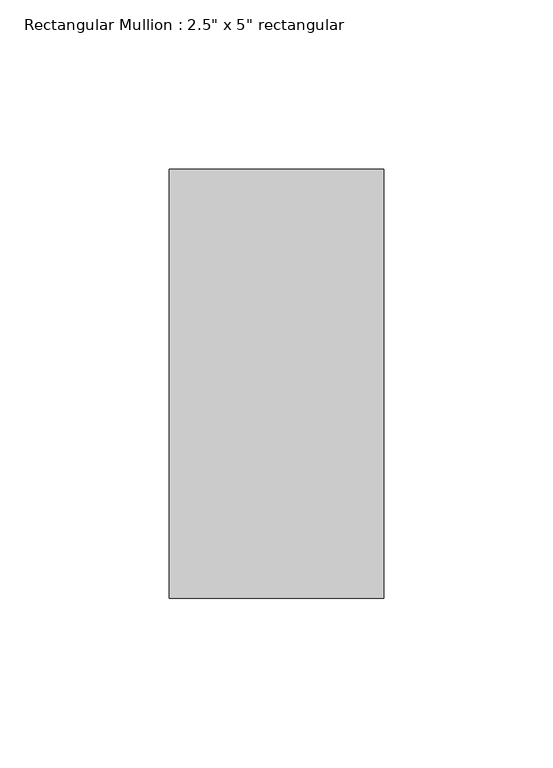
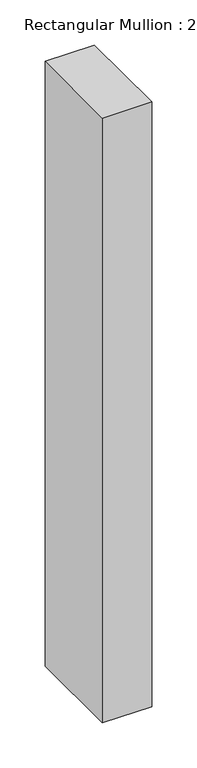
"""IFC4 building model written with IfcOpenShell, lengths in millimetres: member geometry."""

from ifc_helpers import new_model, si_unit, frame, origin, place, context, project, spatial, polyline, outline, extrude, source, transform, mapped, element, save


def member_8dafe1b6(model_context):
    return source(origin(), model_context, "Body", "SweptSolid", [
        extrude(outline(polyline([(31.75, 63.5), (31.75, -63.5), (-31.75, -63.5), (-31.75, 63.5), (31.75, 63.5)])), frame((0.0, 0.0, -820.3881029), z_axis=(0.0, 0.0, 1.0), x_axis=(1.0, 0.0, 0.0)), (0.0, 0.0, 1.0), 820.3881029),
    ])


if __name__ == "__main__":
    model = new_model("IFC4")
    model_context = context("Model", 3, world=origin())
    ifc_project = project(units=[si_unit("LENGTHUNIT", "METRE", prefix="MILLI")], contexts=[model_context])
    site = spatial("IfcSite", under=ifc_project)
    building = spatial("IfcBuilding", under=site)
    placement = place(None, origin())
    member_shape = member_8dafe1b6(model_context)
    element("IfcMember", 1, ObjectType="Rectangular Mullion : 2.5\" x 5\" rectangular", at=placement, inside=building, context=model_context, shape_type="MappedRepresentation", body=[
        mapped(member_shape, transform((0.0, 0.0, 0.0), x_axis=(1.0, 0.0, 0.0), y_axis=(0.0, 1.0, 0.0), z_axis=(0.0, 0.0, 1.0))),
    ])
    save(model, "model.ifc")

# Revit data of these elements
# Type "Rectangular Mullion : 2.5\" x 5\" rectangular"
#   built-in parameter 1007304 = 0.416667 (stored number, unit not read)
#   built-in parameter 1007301 = 0.104167 (stored number, unit not read)
#   built-in parameter 1007300 = 0.104167 (stored number, unit not read)
# Element 1 (IfcMember, "Rectangular Mullion : 2.5\" x 5\" rectangular")
#   Materials on its faces: "Aluminum"
# Materials
#   "Aluminum": class "Metal", colour RGB 247 247 247, transparency 0, Description = "Aluminum 6061", Cost = 0
